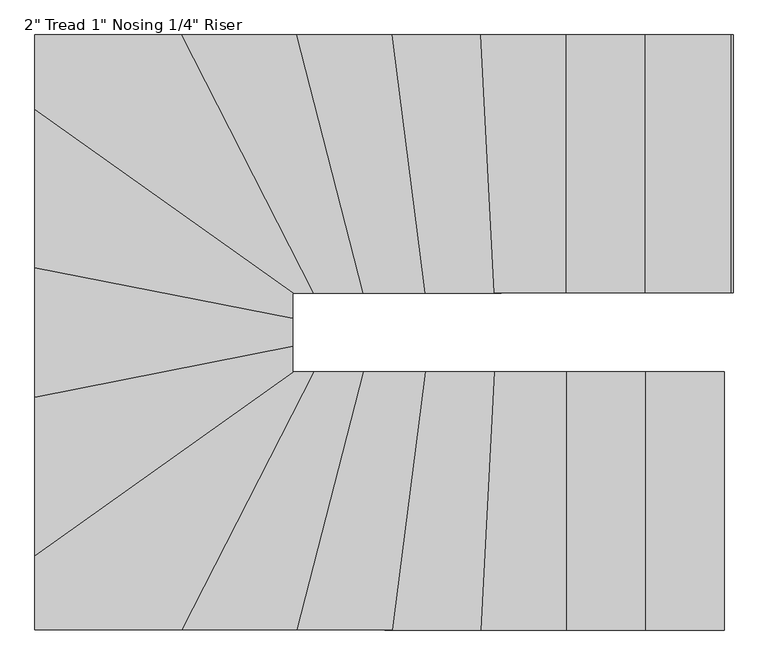
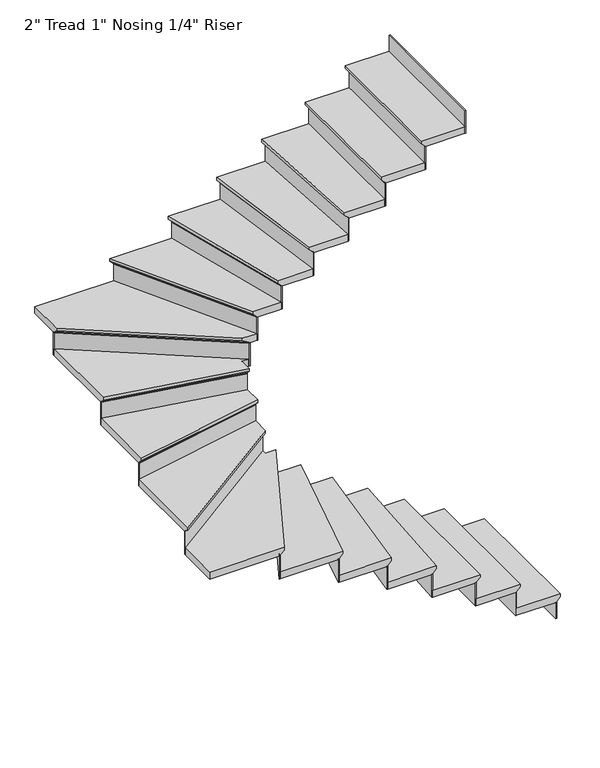
"""IFC4 building model written with IfcOpenShell, lengths in millimetres: stair flight geometry."""

from ifc_helpers import new_model, si_unit, origin, place, context, project, spatial, faceted_brep, source, transform, mapped, element, save


def stair_flight_8889bdd5(model_context):
    return source(origin(), model_context, "Body", "Brep", [
        faceted_brep([(-1783.4132248, -345.7070853, 9751.4833333), (-1783.4132248, -345.7070853, 9770.5333333), (-1783.4132248, -1260.1070853, 9770.5333333), (-1783.4132248, -1260.1070853, 9751.4833333), (-1808.8132248, -345.7070853, 9726.0833333), (-1808.8132248, -1260.1070853, 9726.0833333), (-2088.2132248, -345.7070853, 9770.5333333), (-2088.2132248, -1260.1070853, 9770.5333333), (-1808.8132248, -1260.1070853, 9719.7333333), (-2088.2132248, -1260.1070853, 9719.7333333), (-2088.2132248, -345.7070853, 9719.7333333), (-1808.8132248, -345.7070853, 9719.7333333)], [[[0, 1, 2, 3]], [[4, 0, 3, 5]], [[2, 1, 6, 7]], [[8, 9, 10, 11]], [[2, 7, 9, 8, 5, 3]], [[8, 11, 4, 5]], [[6, 1, 0, 4, 11, 10]], [[7, 6, 10, 9]]]),
        faceted_brep([(-1808.8132248, -345.7070853, 9719.7333333), (-1808.8132248, -345.7070853, 9601.2), (-1815.1632248, -345.7070853, 9601.2), (-1815.1632248, -345.7070853, 9719.7333333), (-1808.8132248, -1260.1070853, 9719.7333333), (-1815.1632248, -1260.1070853, 9719.7333333), (-1815.1632248, -1260.1070853, 9601.2), (-1808.8132248, -1260.1070853, 9601.2)], [[[0, 1, 2, 3]], [[4, 5, 6, 7]], [[1, 0, 4, 7]], [[2, 1, 7, 6]], [[3, 2, 6, 5]], [[0, 3, 5, 4]]]),
        faceted_brep([(-2088.2132248, -345.7070853, 9889.0666667), (-2088.2132248, -345.7070853, 9719.7333333), (-2094.5632248, -345.7070853, 9719.7333333), (-2094.5632248, -345.7070853, 9889.0666667), (-2088.2132248, -1260.1070853, 9889.0666667), (-2094.5632248, -1260.1070853, 9889.0666667), (-2094.5632248, -1260.1070853, 9719.7333333), (-2088.2132248, -1260.1070853, 9719.7333333)], [[[0, 1, 2, 3]], [[4, 5, 6, 7]], [[1, 0, 4, 7]], [[2, 1, 7, 6]], [[3, 2, 6, 5]], [[0, 3, 5, 4]]]),
        faceted_brep([(-2062.8132248, -1260.1070853, 9939.8666667), (-2062.8132248, -345.7070853, 9939.8666667), (-2367.6132248, -345.7070853, 9939.8666667), (-2367.6132248, -1260.1070853, 9939.8666667), (-2088.2132248, -1260.1070853, 9889.0666667), (-2367.6132248, -1260.1070853, 9889.0666667), (-2367.6132248, -345.7070853, 9889.0666667), (-2088.2132248, -345.7070853, 9889.0666667), (-2088.2132248, -1260.1070853, 9895.4166667), (-2062.8132248, -1260.1070853, 9920.8166667), (-2088.2132248, -345.7070853, 9895.4166667), (-2062.8132248, -345.7070853, 9920.8166667)], [[[0, 1, 2, 3]], [[4, 5, 6, 7]], [[0, 3, 5, 4, 8, 9]], [[4, 7, 10, 8]], [[2, 1, 11, 10, 7, 6]], [[3, 2, 6, 5]], [[11, 1, 0, 9]], [[10, 11, 9, 8]]]),
        faceted_brep([(-2367.6132248, -345.7070853, 10058.4), (-2367.6132248, -345.7070853, 9889.0666667), (-2373.9632248, -345.7070853, 9889.0666667), (-2373.9632248, -345.7070853, 10058.4), (-2367.6132248, -1260.1070853, 10058.4), (-2373.9632248, -1260.1070853, 10058.4), (-2373.9632248, -1260.1070853, 9889.0666667), (-2367.6132248, -1260.1070853, 9889.0666667)], [[[0, 1, 2, 3]], [[4, 5, 6, 7]], [[1, 0, 4, 7]], [[2, 1, 7, 6]], [[3, 2, 6, 5]], [[0, 3, 5, 4]]]),
        faceted_brep([(-2342.2132248, -1260.1070853, 10109.2), (-2342.2132248, -345.7070853, 10109.2), (-2623.2803863, -345.7070853, 10109.2), (-2670.8146567, -1260.1070853, 10109.2), (-2367.6132248, -1260.1070853, 10058.4), (-2670.8146567, -1260.1070853, 10058.4), (-2623.2803863, -345.7070853, 10058.4), (-2367.6132248, -345.7070853, 10058.4), (-2367.6132248, -1260.1070853, 10064.75), (-2342.2132248, -1260.1070853, 10090.15), (-2367.6132248, -345.7070853, 10064.75), (-2342.2132248, -345.7070853, 10090.15)], [[[0, 1, 2, 3]], [[4, 5, 6, 7]], [[0, 3, 5, 4, 8, 9]], [[4, 7, 10, 8]], [[2, 1, 11, 10, 7, 6]], [[3, 2, 6, 5]], [[11, 1, 0, 9]], [[10, 11, 9, 8]]]),
        faceted_brep([(-2623.2803863, -345.7070853, 10227.7333333), (-2623.2803863, -345.7070853, 10058.4), (-2629.6389604, -345.7070853, 10058.4), (-2629.6389604, -345.7070853, 10227.7333333), (-2670.8146567, -1260.1070853, 10227.7333333), (-2677.1732308, -1260.1070853, 10227.7333333), (-2677.1732308, -1260.1070853, 10058.4), (-2670.8146567, -1260.1070853, 10058.4)], [[[0, 1, 2, 3]], [[4, 5, 6, 7]], [[1, 0, 4, 7]], [[2, 1, 7, 6]], [[3, 2, 6, 5]], [[0, 3, 5, 4]]]),
        faceted_brep([(-2645.38036, -1260.1070853, 10278.5333333), (-2597.8460896, -345.7070853, 10278.5333333), (-2867.4470861, -345.7070853, 10278.5333333), (-2985.8031378, -1260.1070853, 10278.5333333), (-2670.8146567, -1260.1070853, 10227.7333333), (-2985.8031378, -1260.1070853, 10227.7333333), (-2867.4470861, -345.7070853, 10227.7333333), (-2623.2803863, -345.7070853, 10227.7333333), (-2670.8146567, -1260.1070853, 10234.0833333), (-2645.38036, -1260.1070853, 10259.4833333), (-2623.2803863, -345.7070853, 10234.0833333), (-2597.8460896, -345.7070853, 10259.4833333)], [[[0, 1, 2, 3]], [[4, 5, 6, 7]], [[0, 3, 5, 4, 8, 9]], [[4, 7, 10, 8]], [[2, 1, 11, 10, 7, 6]], [[3, 2, 6, 5]], [[11, 1, 0, 9]], [[10, 11, 9, 8]]]),
        faceted_brep([(-2867.4470861, -345.7070853, 10397.0666667), (-2867.4470861, -345.7070853, 10227.7333333), (-2873.8500579, -345.7070853, 10227.7333333), (-2873.8500579, -345.7070853, 10397.0666667), (-2985.8031378, -1260.1070853, 10397.0666667), (-2992.2061095, -1260.1070853, 10397.0666667), (-2992.2061095, -1260.1070853, 10227.7333333), (-2985.8031378, -1260.1070853, 10227.7333333)], [[[0, 1, 2, 3]], [[4, 5, 6, 7]], [[1, 0, 4, 7]], [[2, 1, 7, 6]], [[3, 2, 6, 5]], [[0, 3, 5, 4]]]),
        faceted_brep([(-2960.1912506, -1260.1070853, 10447.8666667), (-2841.835199, -345.7070853, 10447.8666667), (-3089.0743086, -345.7070853, 10447.8666667), (-3324.204756, -1260.1070853, 10447.8666667), (-2985.8031378, -1260.1070853, 10397.0666667), (-3324.204756, -1260.1070853, 10397.0666667), (-3089.0743086, -345.7070853, 10397.0666667), (-2867.4470861, -345.7070853, 10397.0666667), (-2985.8031378, -1260.1070853, 10403.4166667), (-2960.1912506, -1260.1070853, 10428.8166667), (-2867.4470861, -345.7070853, 10403.4166667), (-2841.835199, -345.7070853, 10428.8166667)], [[[0, 1, 2, 3]], [[4, 5, 6, 7]], [[0, 3, 5, 4, 8, 9]], [[4, 7, 10, 8]], [[2, 1, 11, 10, 7, 6]], [[3, 2, 6, 5]], [[11, 1, 0, 9]], [[10, 11, 9, 8]]]),
        faceted_brep([(-3089.0743086, -345.7070853, 10566.4), (-3089.0743086, -345.7070853, 10397.0666667), (-3095.6308854, -345.7070853, 10397.0666667), (-3095.6308854, -345.7070853, 10566.4), (-3324.204756, -1260.1070853, 10566.4), (-3330.7613329, -1260.1070853, 10566.4), (-3330.7613329, -1260.1070853, 10397.0666667), (-3324.204756, -1260.1070853, 10397.0666667)], [[[0, 1, 2, 3]], [[4, 5, 6, 7]], [[1, 0, 4, 7]], [[2, 1, 7, 6]], [[3, 2, 6, 5]], [[0, 3, 5, 4]]]),
        faceted_brep([(-3297.9784485, -1260.1070853, 10617.2), (-3062.8480011, -345.7070853, 10617.2), (-3265.4209447, -345.7070853, 10617.2), (-3734.245566, -1260.1070853, 10617.2), (-3324.204756, -1260.1070853, 10566.4), (-3734.245566, -1260.1070853, 10566.4), (-3265.4209447, -345.7070853, 10566.4), (-3089.0743086, -345.7070853, 10566.4), (-3324.204756, -1260.1070853, 10572.75), (-3297.9784485, -1260.1070853, 10598.15), (-3089.0743086, -345.7070853, 10572.75), (-3062.8480011, -345.7070853, 10598.15)], [[[0, 1, 2, 3]], [[4, 5, 6, 7]], [[0, 3, 5, 4, 8, 9]], [[4, 7, 10, 8]], [[2, 1, 11, 10, 7, 6]], [[3, 2, 6, 5]], [[11, 1, 0, 9]], [[10, 11, 9, 8]]]),
        faceted_brep([(-3265.4209447, -345.7070853, 10735.7333333), (-3265.4209447, -345.7070853, 10566.4), (-3272.5569278, -345.7070853, 10566.4), (-3272.5569278, -345.7070853, 10735.7333333), (-3734.245566, -1260.1070853, 10735.7333333), (-3741.3815491, -1260.1070853, 10735.7333333), (-3741.3815491, -1260.1070853, 10566.4), (-3734.245566, -1260.1070853, 10566.4)], [[[0, 1, 2, 3]], [[4, 5, 6, 7]], [[1, 0, 4, 7]], [[2, 1, 7, 6]], [[3, 2, 6, 5]], [[0, 3, 5, 4]]]),
        faceted_brep([(-4225.5449167, -966.4259516, 10786.5333333), (-4225.5449167, -1260.1070853, 10786.5333333), (-3705.7016335, -1260.1070853, 10786.5333333), (-3236.8770121, -345.7070853, 10786.5333333), (-3311.1449167, -345.7070853, 10786.5333333), (-3311.1449167, -316.1520025, 10786.5333333), (-4225.5449167, -1260.1070853, 10735.7333333), (-4225.5449167, -966.4259516, 10735.7333333), (-3311.1449167, -316.1520025, 10735.7333333), (-3311.1449167, -345.7070853, 10735.7333333), (-3265.4209447, -345.7070853, 10735.7333333), (-3734.245566, -1260.1070853, 10735.7333333), (-3734.245566, -1260.1070853, 10742.0833333), (-3705.7016335, -1260.1070853, 10767.4833333), (-3265.4209447, -345.7070853, 10742.0833333), (-3236.8770121, -345.7070853, 10767.4833333)], [[[0, 1, 2, 3, 4, 5]], [[6, 7, 8, 9, 10, 11]], [[1, 0, 7, 6]], [[2, 1, 6, 11, 12, 13]], [[11, 10, 14, 12]], [[4, 3, 15, 14, 10, 9]], [[5, 4, 9, 8]], [[0, 5, 8, 7]], [[15, 3, 2, 13]], [[14, 15, 13, 12]]]),
        faceted_brep([(-3311.1449167, -316.1520025, 10905.0666667), (-3311.1449167, -316.1520025, 10735.7333333), (-3311.1449167, -308.3600277, 10735.7333333), (-3311.1449167, -308.3600277, 10905.0666667), (-4225.5449167, -966.4259516, 10905.0666667), (-4225.5449167, -958.6339768, 10905.0666667), (-4225.5449167, -958.6339768, 10735.7333333), (-4225.5449167, -966.4259516, 10735.7333333)], [[[0, 1, 2, 3]], [[4, 5, 6, 7]], [[1, 0, 4, 7]], [[2, 1, 7, 6]], [[3, 2, 6, 5]], [[0, 3, 5, 4]]]),
        faceted_brep([(-4225.5449167, -997.5938508, 10955.8666667), (-3311.1449167, -347.3199017, 10955.8666667), (-3311.1449167, -229.6979154, 10955.8666667), (-4225.5449167, -409.9387717, 10955.8666667), (-4225.5449167, -966.4259516, 10905.0666667), (-4225.5449167, -409.9387717, 10905.0666667), (-3311.1449167, -229.6979154, 10905.0666667), (-3311.1449167, -316.1520025, 10905.0666667), (-4225.5449167, -966.4259516, 10911.4166667), (-4225.5449167, -997.5938508, 10936.8166667), (-3311.1449167, -316.1520025, 10911.4166667), (-3311.1449167, -347.3199017, 10936.8166667)], [[[0, 1, 2, 3]], [[4, 5, 6, 7]], [[0, 3, 5, 4, 8, 9]], [[4, 7, 10, 8]], [[2, 1, 11, 10, 7, 6]], [[3, 2, 6, 5]], [[11, 1, 0, 9]], [[10, 11, 9, 8]]]),
        faceted_brep([(-3311.1449167, -229.6979154, 11074.4), (-3311.1449167, -229.6979154, 10905.0666667), (-3311.1449167, -223.22573, 10905.0666667), (-3311.1449167, -223.22573, 11074.4), (-4225.5449167, -409.9387717, 11074.4), (-4225.5449167, -403.4665863, 11074.4), (-4225.5449167, -403.4665863, 10905.0666667), (-4225.5449167, -409.9387717, 10905.0666667)], [[[0, 1, 2, 3]], [[4, 5, 6, 7]], [[1, 0, 4, 7]], [[2, 1, 7, 6]], [[3, 2, 6, 5]], [[0, 3, 5, 4]]]),
        faceted_brep([(-4225.5449167, -435.8275135, 11125.2), (-3311.1449167, -255.5866572, 11125.2), (-3311.1449167, -130.5387717, 11125.2), (-4225.5449167, 49.7020846, 11125.2), (-4225.5449167, -409.9387717, 11074.4), (-4225.5449167, 49.7020846, 11074.4), (-3311.1449167, -130.5387717, 11074.4), (-3311.1449167, -229.6979154, 11074.4), (-4225.5449167, -409.9387717, 11080.75), (-4225.5449167, -435.8275135, 11106.15), (-3311.1449167, -229.6979154, 11080.75), (-3311.1449167, -255.5866572, 11106.15)], [[[0, 1, 2, 3]], [[4, 5, 6, 7]], [[0, 3, 5, 4, 8, 9]], [[4, 7, 10, 8]], [[2, 1, 11, 10, 7, 6]], [[3, 2, 6, 5]], [[11, 1, 0, 9]], [[10, 11, 9, 8]]]),
        faceted_brep([(-3311.1449167, -130.5387717, 11243.7333333), (-3311.1449167, -130.5387717, 11074.4), (-3311.1449167, -124.0665863, 11074.4), (-3311.1449167, -124.0665863, 11243.7333333), (-4225.5449167, 49.7020846, 11243.7333333), (-4225.5449167, 56.17427, 11243.7333333), (-4225.5449167, 56.17427, 11074.4), (-4225.5449167, 49.7020846, 11074.4)], [[[0, 1, 2, 3]], [[4, 5, 6, 7]], [[1, 0, 4, 7]], [[2, 1, 7, 6]], [[3, 2, 6, 5]], [[0, 3, 5, 4]]]),
        faceted_brep([(-4225.5449167, 23.8133428, 11294.5333333), (-3311.1449167, -156.4275135, 11294.5333333), (-3311.1449167, -66.3070853, 11294.5333333), (-3265.0494422, -66.3070853, 11294.5333333), (-4225.5449167, 616.7475793, 11294.5333333), (-4225.5449167, 49.7020846, 11243.7333333), (-4225.5449167, 616.7475793, 11243.7333333), (-3265.0494422, -66.3070853, 11243.7333333), (-3311.1449167, -66.3070853, 11243.7333333), (-3311.1449167, -130.5387717, 11243.7333333), (-4225.5449167, 49.7020846, 11250.0833333), (-4225.5449167, 23.8133428, 11275.4833333), (-3311.1449167, -130.5387717, 11250.0833333), (-3311.1449167, -156.4275135, 11275.4833333)], [[[0, 1, 2, 3, 4]], [[5, 6, 7, 8, 9]], [[0, 4, 6, 5, 10, 11]], [[5, 9, 12, 10]], [[2, 1, 13, 12, 9, 8]], [[3, 2, 8, 7]], [[4, 3, 7, 6]], [[13, 1, 0, 11]], [[12, 13, 11, 10]]]),
        faceted_brep([(-3265.0494422, -66.3070853, 11413.0666667), (-3265.0494422, -66.3070853, 11243.7333333), (-3254.0925497, -66.3070853, 11243.7333333), (-3254.0925497, -66.3070853, 11413.0666667), (-4225.5449167, 616.7475793, 11413.0666667), (-4225.5449167, 624.5395541, 11413.0666667), (-4225.5449167, 624.5395541, 11243.7333333), (-4225.5449167, 616.7475793, 11243.7333333)], [[[0, 1, 2, 3]], [[4, 5, 6, 7]], [[1, 0, 4, 7]], [[2, 1, 7, 6]], [[3, 2, 6, 5]], [[0, 3, 5, 4]]]),
        faceted_brep([(-3677.1577009, 848.0929147, 11463.8666667), (-4225.5449167, 848.0929147, 11463.8666667), (-4225.5449167, 585.5796802, 11463.8666667), (-3308.8770121, -66.3070853, 11463.8666667), (-3208.3330796, -66.3070853, 11463.8666667), (-4225.5449167, 848.0929147, 11413.0666667), (-3677.1577009, 848.0929147, 11413.0666667), (-3208.3330796, -66.3070853, 11413.0666667), (-3265.0494422, -66.3070853, 11413.0666667), (-4225.5449167, 616.7475793, 11413.0666667), (-4225.5449167, 616.7475793, 11419.4166667), (-4225.5449167, 585.5796802, 11444.8166667), (-3265.0494422, -66.3070853, 11419.4166667), (-3308.8770121, -66.3070853, 11444.8166667)], [[[0, 1, 2, 3, 4]], [[5, 6, 7, 8, 9]], [[1, 0, 6, 5]], [[2, 1, 5, 9, 10, 11]], [[9, 8, 12, 10]], [[4, 3, 13, 12, 8, 7]], [[0, 4, 7, 6]], [[13, 3, 2, 11]], [[12, 13, 11, 10]]]),
        faceted_brep([(-3208.3330796, -66.3070853, 11582.4), (-3208.3330796, -66.3070853, 11413.0666667), (-3201.1970965, -66.3070853, 11413.0666667), (-3201.1970965, -66.3070853, 11582.4), (-3677.1577009, 848.0929147, 11582.4), (-3670.0217178, 848.0929147, 11582.4), (-3670.0217178, 848.0929147, 11413.0666667), (-3677.1577009, 848.0929147, 11413.0666667)], [[[0, 1, 2, 3]], [[4, 5, 6, 7]], [[1, 0, 4, 7]], [[2, 1, 7, 6]], [[3, 2, 6, 5]], [[0, 3, 5, 4]]]),
        faceted_brep([(-3705.7016335, 848.0929147, 11633.2), (-3236.8770121, -66.3070853, 11633.2), (-3036.6216937, -66.3070853, 11633.2), (-3271.7521411, 848.0929147, 11633.2), (-3677.1577009, 848.0929147, 11582.4), (-3271.7521411, 848.0929147, 11582.4), (-3036.6216937, -66.3070853, 11582.4), (-3208.3330796, -66.3070853, 11582.4), (-3677.1577009, 848.0929147, 11588.75), (-3705.7016335, 848.0929147, 11614.15), (-3208.3330796, -66.3070853, 11588.75), (-3236.8770121, -66.3070853, 11614.15)], [[[0, 1, 2, 3]], [[4, 5, 6, 7]], [[0, 3, 5, 4, 8, 9]], [[4, 7, 10, 8]], [[2, 1, 11, 10, 7, 6]], [[3, 2, 6, 5]], [[11, 1, 0, 9]], [[10, 11, 9, 8]]]),
        faceted_brep([(-3036.6216937, -66.3070853, 11751.7333333), (-3036.6216937, -66.3070853, 11582.4), (-3030.0651168, -66.3070853, 11582.4), (-3030.0651168, -66.3070853, 11751.7333333), (-3271.7521411, 848.0929147, 11751.7333333), (-3265.1955642, 848.0929147, 11751.7333333), (-3265.1955642, 848.0929147, 11582.4), (-3271.7521411, 848.0929147, 11582.4)], [[[0, 1, 2, 3]], [[4, 5, 6, 7]], [[1, 0, 4, 7]], [[2, 1, 7, 6]], [[3, 2, 6, 5]], [[0, 3, 5, 4]]]),
        faceted_brep([(-3297.9784485, 848.0929147, 11802.5333333), (-3062.8480011, -66.3070853, 11802.5333333), (-2816.2233119, -66.3070853, 11802.5333333), (-2934.5793635, 848.0929147, 11802.5333333), (-3271.7521411, 848.0929147, 11751.7333333), (-2934.5793635, 848.0929147, 11751.7333333), (-2816.2233119, -66.3070853, 11751.7333333), (-3036.6216937, -66.3070853, 11751.7333333), (-3271.7521411, 848.0929147, 11758.0833333), (-3297.9784485, 848.0929147, 11783.4833333), (-3036.6216937, -66.3070853, 11758.0833333), (-3062.8480011, -66.3070853, 11783.4833333)], [[[0, 1, 2, 3]], [[4, 5, 6, 7]], [[0, 3, 5, 4, 8, 9]], [[4, 7, 10, 8]], [[2, 1, 11, 10, 7, 6]], [[3, 2, 6, 5]], [[11, 1, 0, 9]], [[10, 11, 9, 8]]]),
        faceted_brep([(-2816.2233119, -66.3070853, 11921.0666667), (-2816.2233119, -66.3070853, 11751.7333333), (-2809.8203401, -66.3070853, 11751.7333333), (-2809.8203401, -66.3070853, 11921.0666667), (-2934.5793635, 848.0929147, 11921.0666667), (-2928.1763918, 848.0929147, 11921.0666667), (-2928.1763918, 848.0929147, 11751.7333333), (-2934.5793635, 848.0929147, 11751.7333333)], [[[0, 1, 2, 3]], [[4, 5, 6, 7]], [[1, 0, 4, 7]], [[2, 1, 7, 6]], [[3, 2, 6, 5]], [[0, 3, 5, 4]]]),
        faceted_brep([(-2960.1912506, 848.0929147, 11971.8666667), (-2841.835199, -66.3070853, 11971.8666667), (-2572.411793, -66.3070853, 11971.8666667), (-2619.9460634, 848.0929147, 11971.8666667), (-2934.5793635, 848.0929147, 11921.0666667), (-2619.9460634, 848.0929147, 11921.0666667), (-2572.411793, -66.3070853, 11921.0666667), (-2816.2233119, -66.3070853, 11921.0666667), (-2934.5793635, 848.0929147, 11927.4166667), (-2960.1912506, 848.0929147, 11952.8166667), (-2816.2233119, -66.3070853, 11927.4166667), (-2841.835199, -66.3070853, 11952.8166667)], [[[0, 1, 2, 3]], [[4, 5, 6, 7]], [[0, 3, 5, 4, 8, 9]], [[4, 7, 10, 8]], [[2, 1, 11, 10, 7, 6]], [[3, 2, 6, 5]], [[11, 1, 0, 9]], [[10, 11, 9, 8]]]),
        faceted_brep([(-2572.411793, -66.3070853, 12090.4), (-2572.411793, -66.3070853, 11921.0666667), (-2566.0532188, -66.3070853, 11921.0666667), (-2566.0532188, -66.3070853, 12090.4), (-2619.9460634, 848.0929147, 12090.4), (-2613.5874892, 848.0929147, 12090.4), (-2613.5874892, 848.0929147, 11921.0666667), (-2619.9460634, 848.0929147, 11921.0666667)], [[[0, 1, 2, 3]], [[4, 5, 6, 7]], [[1, 0, 4, 7]], [[2, 1, 7, 6]], [[3, 2, 6, 5]], [[0, 3, 5, 4]]]),
        faceted_brep([(-2645.38036, 848.0929147, 12141.2), (-2597.8460896, -66.3070853, 12141.2), (-2316.8132248, -66.3070853, 12141.2), (-2316.8132248, 848.0929147, 12141.2), (-2619.9460634, 848.0929147, 12090.4), (-2316.8132248, 848.0929147, 12090.4), (-2316.8132248, -66.3070853, 12090.4), (-2572.411793, -66.3070853, 12090.4), (-2619.9460634, 848.0929147, 12096.75), (-2645.38036, 848.0929147, 12122.15), (-2572.411793, -66.3070853, 12096.75), (-2597.8460896, -66.3070853, 12122.15)], [[[0, 1, 2, 3]], [[4, 5, 6, 7]], [[0, 3, 5, 4, 8, 9]], [[4, 7, 10, 8]], [[2, 1, 11, 10, 7, 6]], [[3, 2, 6, 5]], [[11, 1, 0, 9]], [[10, 11, 9, 8]]]),
        faceted_brep([(-2316.8132248, -66.3070853, 12259.7333333), (-2316.8132248, -66.3070853, 12090.4), (-2310.4632248, -66.3070853, 12090.4), (-2310.4632248, -66.3070853, 12259.7333333), (-2316.8132248, 848.0929147, 12259.7333333), (-2310.4632248, 848.0929147, 12259.7333333), (-2310.4632248, 848.0929147, 12090.4), (-2316.8132248, 848.0929147, 12090.4)], [[[0, 1, 2, 3]], [[4, 5, 6, 7]], [[1, 0, 4, 7]], [[2, 1, 7, 6]], [[3, 2, 6, 5]], [[0, 3, 5, 4]]]),
        faceted_brep([(-2342.2132248, 848.0929147, 12310.5333333), (-2342.2132248, -66.3070853, 12310.5333333), (-2037.4132248, -66.3070853, 12310.5333333), (-2037.4132248, 848.0929147, 12310.5333333), (-2316.8132248, 848.0929147, 12259.7333333), (-2037.4132248, 848.0929147, 12259.7333333), (-2037.4132248, -66.3070853, 12259.7333333), (-2316.8132248, -66.3070853, 12259.7333333), (-2316.8132248, 848.0929147, 12266.0833333), (-2342.2132248, 848.0929147, 12291.4833333), (-2316.8132248, -66.3070853, 12266.0833333), (-2342.2132248, -66.3070853, 12291.4833333)], [[[0, 1, 2, 3]], [[4, 5, 6, 7]], [[0, 3, 5, 4, 8, 9]], [[4, 7, 10, 8]], [[2, 1, 11, 10, 7, 6]], [[3, 2, 6, 5]], [[11, 1, 0, 9]], [[10, 11, 9, 8]]]),
        faceted_brep([(-2037.4132248, -66.3070853, 12429.0666667), (-2037.4132248, -66.3070853, 12259.7333333), (-2031.0632248, -66.3070853, 12259.7333333), (-2031.0632248, -66.3070853, 12429.0666667), (-2037.4132248, 848.0929147, 12429.0666667), (-2031.0632248, 848.0929147, 12429.0666667), (-2031.0632248, 848.0929147, 12259.7333333), (-2037.4132248, 848.0929147, 12259.7333333)], [[[0, 1, 2, 3]], [[4, 5, 6, 7]], [[1, 0, 4, 7]], [[2, 1, 7, 6]], [[3, 2, 6, 5]], [[0, 3, 5, 4]]]),
        faceted_brep([(-1758.0132248, -66.3070853, 12598.4), (-1758.0132248, -66.3070853, 12429.0666667), (-1751.6632248, -66.3070853, 12429.0666667), (-1751.6632248, -66.3070853, 12598.4), (-1758.0132248, 848.0929147, 12598.4), (-1751.6632248, 848.0929147, 12598.4), (-1751.6632248, 848.0929147, 12429.0666667), (-1758.0132248, 848.0929147, 12429.0666667)], [[[0, 1, 2, 3]], [[4, 5, 6, 7]], [[1, 0, 4, 7]], [[2, 1, 7, 6]], [[3, 2, 6, 5]], [[0, 3, 5, 4]]]),
        faceted_brep([(-2062.8132248, 848.0929147, 12479.8666667), (-2062.8132248, -66.3070853, 12479.8666667), (-1758.0132248, -66.3070853, 12479.8666667), (-1758.0132248, 848.0929147, 12479.8666667), (-2037.4132248, 848.0929147, 12429.0666667), (-1758.0132248, 848.0929147, 12429.0666667), (-1758.0132248, -66.3070853, 12429.0666667), (-2037.4132248, -66.3070853, 12429.0666667), (-2037.4132248, 848.0929147, 12435.4166667), (-2062.8132248, 848.0929147, 12460.8166667), (-2037.4132248, -66.3070853, 12435.4166667), (-2062.8132248, -66.3070853, 12460.8166667)], [[[0, 1, 2, 3]], [[4, 5, 6, 7]], [[0, 3, 5, 4, 8, 9]], [[4, 7, 10, 8]], [[2, 1, 11, 10, 7, 6]], [[3, 2, 6, 5]], [[11, 1, 0, 9]], [[10, 11, 9, 8]]]),
    ])


if __name__ == "__main__":
    model = new_model("IFC4")
    model_context = context("Model", 3, world=origin())
    ifc_project = project(units=[si_unit("LENGTHUNIT", "METRE", prefix="MILLI")], contexts=[model_context])
    site = spatial("IfcSite", under=ifc_project)
    building = spatial("IfcBuilding", under=site)
    placement = place(None, origin())
    stair_flight_shape = stair_flight_8889bdd5(model_context)
    element("IfcStairFlight", 1, ObjectType="2\" Tread 1\" Nosing 1/4\" Riser", at=placement, inside=building, context=model_context, shape_type="MappedRepresentation", body=[
        mapped(stair_flight_shape, transform((0.0, 0.0, 0.0), x_axis=(1.0, 0.0, 0.0), y_axis=(0.0, 1.0, 0.0), z_axis=(0.0, 0.0, 1.0))),
    ])
    save(model, "model.ifc")
